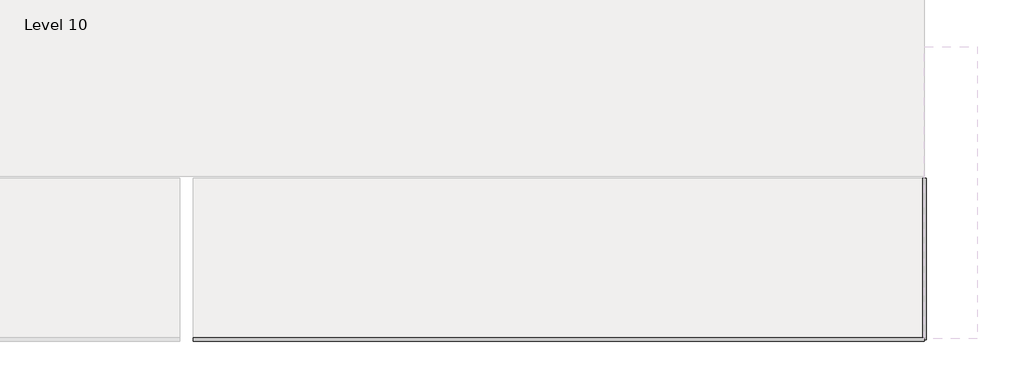
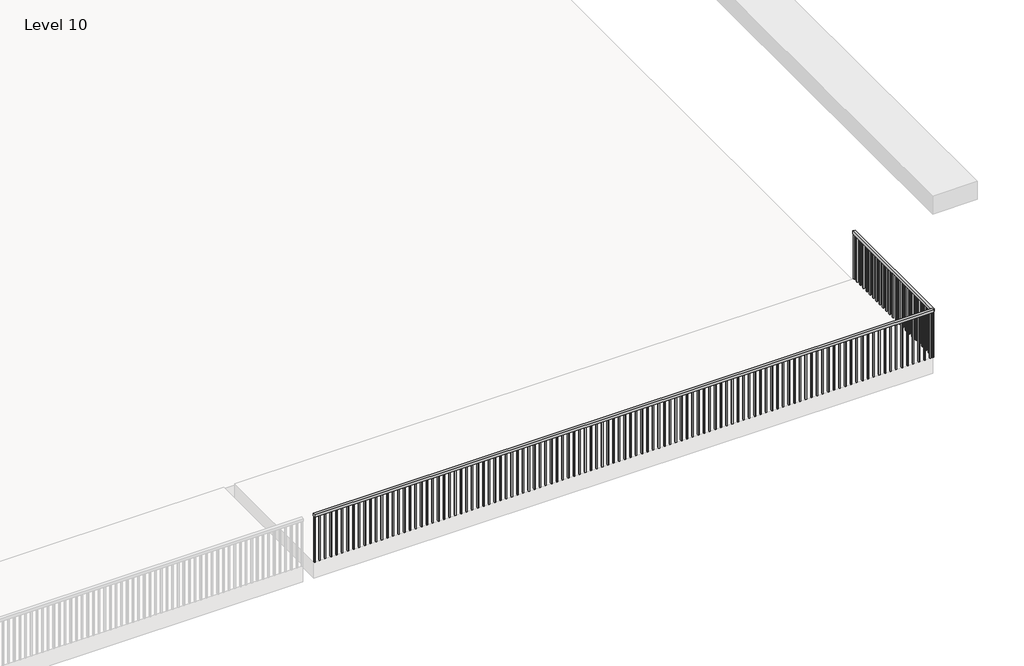
# One storey, part 2 of 5: 2 railings.
"""IFC4 building model written with IfcOpenShell, lengths in millimetres."""

from ifc_helpers import new_model, si_unit, frame, origin, place, context, project, spatial, polyline, outline, extrude, element, save

model = new_model("IFC4")

# Units and contexts
model_context = context("Model", 3, world=origin())
ifc_project = project(units=[si_unit("LENGTHUNIT", "METRE", prefix="MILLI")], contexts=[model_context])

# Site, building, storey
site = spatial("IfcSite", under=ifc_project)
building = spatial("IfcBuilding", under=site)
storey = spatial("IfcBuildingStorey", under=building, Name="Level 10", Elevation=12496.8)

# Railings
placement = place(None, origin())
element("IfcRailing", 1, ObjectType="Handrail - Rectangular", at=placement, inside=storey, context=model_context, shape_type="SweptSolid", body=[
    extrude(outline(polyline([(2981.3361222, -12911.7749501), (2981.3361222, -12860.9749501), (14106.5361222, -12860.9749501), (14106.5361222, -12911.7749501), (2981.3361222, -12911.7749501)])), frame((0.0, 0.0, 13360.4), z_axis=(0.0, 0.0, 1.0), x_axis=(1.0, 0.0, 0.0)), (0.0, 0.0, 1.0), 50.8),
    extrude(outline(polyline([(14046.2111222, -12895.8999501), (14046.2111222, -12876.8499501), (14065.2611222, -12876.8499501), (14065.2611222, -12895.8999501), (14046.2111222, -12895.8999501)])), frame((0.0, 0.0, 12496.8), z_axis=(0.0, 0.0, 1.0), x_axis=(1.0, 0.0, 0.0)), (0.0, 0.0, 1.0), 863.6),
    extrude(outline(polyline([(13944.6111222, -12895.8999501), (13944.6111222, -12876.8499501), (13963.6611222, -12876.8499501), (13963.6611222, -12895.8999501), (13944.6111222, -12895.8999501)])), frame((0.0, 0.0, 12496.8), z_axis=(0.0, 0.0, 1.0), x_axis=(1.0, 0.0, 0.0)), (0.0, 0.0, 1.0), 863.6),
    extrude(outline(polyline([(13843.0111222, -12895.8999501), (13843.0111222, -12876.8499501), (13862.0611222, -12876.8499501), (13862.0611222, -12895.8999501), (13843.0111222, -12895.8999501)])), frame((0.0, 0.0, 12496.8), z_axis=(0.0, 0.0, 1.0), x_axis=(1.0, 0.0, 0.0)), (0.0, 0.0, 1.0), 863.6),
    extrude(outline(polyline([(13741.4111222, -12895.8999501), (13741.4111222, -12876.8499501), (13760.4611222, -12876.8499501), (13760.4611222, -12895.8999501), (13741.4111222, -12895.8999501)])), frame((0.0, 0.0, 12496.8), z_axis=(0.0, 0.0, 1.0), x_axis=(1.0, 0.0, 0.0)), (0.0, 0.0, 1.0), 863.6),
    extrude(outline(polyline([(13639.8111222, -12895.8999501), (13639.8111222, -12876.8499501), (13658.8611222, -12876.8499501), (13658.8611222, -12895.8999501), (13639.8111222, -12895.8999501)])), frame((0.0, 0.0, 12496.8), z_axis=(0.0, 0.0, 1.0), x_axis=(1.0, 0.0, 0.0)), (0.0, 0.0, 1.0), 863.6),
    extrude(outline(polyline([(13538.2111222, -12895.8999501), (13538.2111222, -12876.8499501), (13557.2611222, -12876.8499501), (13557.2611222, -12895.8999501), (13538.2111222, -12895.8999501)])), frame((0.0, 0.0, 12496.8), z_axis=(0.0, 0.0, 1.0), x_axis=(1.0, 0.0, 0.0)), (0.0, 0.0, 1.0), 863.6),
    extrude(outline(polyline([(13436.6111222, -12895.8999501), (13436.6111222, -12876.8499501), (13455.6611222, -12876.8499501), (13455.6611222, -12895.8999501), (13436.6111222, -12895.8999501)])), frame((0.0, 0.0, 12496.8), z_axis=(0.0, 0.0, 1.0), x_axis=(1.0, 0.0, 0.0)), (0.0, 0.0, 1.0), 863.6),
    extrude(outline(polyline([(13335.0111222, -12895.8999501), (13335.0111222, -12876.8499501), (13354.0611222, -12876.8499501), (13354.0611222, -12895.8999501), (13335.0111222, -12895.8999501)])), frame((0.0, 0.0, 12496.8), z_axis=(0.0, 0.0, 1.0), x_axis=(1.0, 0.0, 0.0)), (0.0, 0.0, 1.0), 863.6),
    extrude(outline(polyline([(13233.4111222, -12895.8999501), (13233.4111222, -12876.8499501), (13252.4611222, -12876.8499501), (13252.4611222, -12895.8999501), (13233.4111222, -12895.8999501)])), frame((0.0, 0.0, 12496.8), z_axis=(0.0, 0.0, 1.0), x_axis=(1.0, 0.0, 0.0)), (0.0, 0.0, 1.0), 863.6),
    extrude(outline(polyline([(13131.8111222, -12895.8999501), (13131.8111222, -12876.8499501), (13150.8611222, -12876.8499501), (13150.8611222, -12895.8999501), (13131.8111222, -12895.8999501)])), frame((0.0, 0.0, 12496.8), z_axis=(0.0, 0.0, 1.0), x_axis=(1.0, 0.0, 0.0)), (0.0, 0.0, 1.0), 863.6),
    extrude(outline(polyline([(13030.2111222, -12895.8999501), (13030.2111222, -12876.8499501), (13049.2611222, -12876.8499501), (13049.2611222, -12895.8999501), (13030.2111222, -12895.8999501)])), frame((0.0, 0.0, 12496.8), z_axis=(0.0, 0.0, 1.0), x_axis=(1.0, 0.0, 0.0)), (0.0, 0.0, 1.0), 863.6),
    extrude(outline(polyline([(12928.6111222, -12895.8999501), (12928.6111222, -12876.8499501), (12947.6611222, -12876.8499501), (12947.6611222, -12895.8999501), (12928.6111222, -12895.8999501)])), frame((0.0, 0.0, 12496.8), z_axis=(0.0, 0.0, 1.0), x_axis=(1.0, 0.0, 0.0)), (0.0, 0.0, 1.0), 863.6),
    extrude(outline(polyline([(12827.0111222, -12895.8999501), (12827.0111222, -12876.8499501), (12846.0611222, -12876.8499501), (12846.0611222, -12895.8999501), (12827.0111222, -12895.8999501)])), frame((0.0, 0.0, 12496.8), z_axis=(0.0, 0.0, 1.0), x_axis=(1.0, 0.0, 0.0)), (0.0, 0.0, 1.0), 863.6),
    extrude(outline(polyline([(12725.4111222, -12895.8999501), (12725.4111222, -12876.8499501), (12744.4611222, -12876.8499501), (12744.4611222, -12895.8999501), (12725.4111222, -12895.8999501)])), frame((0.0, 0.0, 12496.8), z_axis=(0.0, 0.0, 1.0), x_axis=(1.0, 0.0, 0.0)), (0.0, 0.0, 1.0), 863.6),
    extrude(outline(polyline([(12623.8111222, -12895.8999501), (12623.8111222, -12876.8499501), (12642.8611222, -12876.8499501), (12642.8611222, -12895.8999501), (12623.8111222, -12895.8999501)])), frame((0.0, 0.0, 12496.8), z_axis=(0.0, 0.0, 1.0), x_axis=(1.0, 0.0, 0.0)), (0.0, 0.0, 1.0), 863.6),
    extrude(outline(polyline([(12522.2111222, -12895.8999501), (12522.2111222, -12876.8499501), (12541.2611222, -12876.8499501), (12541.2611222, -12895.8999501), (12522.2111222, -12895.8999501)])), frame((0.0, 0.0, 12496.8), z_axis=(0.0, 0.0, 1.0), x_axis=(1.0, 0.0, 0.0)), (0.0, 0.0, 1.0), 863.6),
    extrude(outline(polyline([(12420.6111222, -12895.8999501), (12420.6111222, -12876.8499501), (12439.6611222, -12876.8499501), (12439.6611222, -12895.8999501), (12420.6111222, -12895.8999501)])), frame((0.0, 0.0, 12496.8), z_axis=(0.0, 0.0, 1.0), x_axis=(1.0, 0.0, 0.0)), (0.0, 0.0, 1.0), 863.6),
    extrude(outline(polyline([(12319.0111222, -12895.8999501), (12319.0111222, -12876.8499501), (12338.0611222, -12876.8499501), (12338.0611222, -12895.8999501), (12319.0111222, -12895.8999501)])), frame((0.0, 0.0, 12496.8), z_axis=(0.0, 0.0, 1.0), x_axis=(1.0, 0.0, 0.0)), (0.0, 0.0, 1.0), 863.6),
    extrude(outline(polyline([(12217.4111222, -12895.8999501), (12217.4111222, -12876.8499501), (12236.4611222, -12876.8499501), (12236.4611222, -12895.8999501), (12217.4111222, -12895.8999501)])), frame((0.0, 0.0, 12496.8), z_axis=(0.0, 0.0, 1.0), x_axis=(1.0, 0.0, 0.0)), (0.0, 0.0, 1.0), 863.6),
    extrude(outline(polyline([(12115.8111222, -12895.8999501), (12115.8111222, -12876.8499501), (12134.8611222, -12876.8499501), (12134.8611222, -12895.8999501), (12115.8111222, -12895.8999501)])), frame((0.0, 0.0, 12496.8), z_axis=(0.0, 0.0, 1.0), x_axis=(1.0, 0.0, 0.0)), (0.0, 0.0, 1.0), 863.6),
    extrude(outline(polyline([(12014.2111222, -12895.8999501), (12014.2111222, -12876.8499501), (12033.2611222, -12876.8499501), (12033.2611222, -12895.8999501), (12014.2111222, -12895.8999501)])), frame((0.0, 0.0, 12496.8), z_axis=(0.0, 0.0, 1.0), x_axis=(1.0, 0.0, 0.0)), (0.0, 0.0, 1.0), 863.6),
    extrude(outline(polyline([(11912.6111222, -12895.8999501), (11912.6111222, -12876.8499501), (11931.6611222, -12876.8499501), (11931.6611222, -12895.8999501), (11912.6111222, -12895.8999501)])), frame((0.0, 0.0, 12496.8), z_axis=(0.0, 0.0, 1.0), x_axis=(1.0, 0.0, 0.0)), (0.0, 0.0, 1.0), 863.6),
    extrude(outline(polyline([(11811.0111222, -12895.8999501), (11811.0111222, -12876.8499501), (11830.0611222, -12876.8499501), (11830.0611222, -12895.8999501), (11811.0111222, -12895.8999501)])), frame((0.0, 0.0, 12496.8), z_axis=(0.0, 0.0, 1.0), x_axis=(1.0, 0.0, 0.0)), (0.0, 0.0, 1.0), 863.6),
    extrude(outline(polyline([(11709.4111222, -12895.8999501), (11709.4111222, -12876.8499501), (11728.4611222, -12876.8499501), (11728.4611222, -12895.8999501), (11709.4111222, -12895.8999501)])), frame((0.0, 0.0, 12496.8), z_axis=(0.0, 0.0, 1.0), x_axis=(1.0, 0.0, 0.0)), (0.0, 0.0, 1.0), 863.6),
    extrude(outline(polyline([(11607.8111222, -12895.8999501), (11607.8111222, -12876.8499501), (11626.8611222, -12876.8499501), (11626.8611222, -12895.8999501), (11607.8111222, -12895.8999501)])), frame((0.0, 0.0, 12496.8), z_axis=(0.0, 0.0, 1.0), x_axis=(1.0, 0.0, 0.0)), (0.0, 0.0, 1.0), 863.6),
    extrude(outline(polyline([(11506.2111222, -12895.8999501), (11506.2111222, -12876.8499501), (11525.2611222, -12876.8499501), (11525.2611222, -12895.8999501), (11506.2111222, -12895.8999501)])), frame((0.0, 0.0, 12496.8), z_axis=(0.0, 0.0, 1.0), x_axis=(1.0, 0.0, 0.0)), (0.0, 0.0, 1.0), 863.6),
    extrude(outline(polyline([(11404.6111222, -12895.8999501), (11404.6111222, -12876.8499501), (11423.6611222, -12876.8499501), (11423.6611222, -12895.8999501), (11404.6111222, -12895.8999501)])), frame((0.0, 0.0, 12496.8), z_axis=(0.0, 0.0, 1.0), x_axis=(1.0, 0.0, 0.0)), (0.0, 0.0, 1.0), 863.6),
    extrude(outline(polyline([(11303.0111222, -12895.8999501), (11303.0111222, -12876.8499501), (11322.0611222, -12876.8499501), (11322.0611222, -12895.8999501), (11303.0111222, -12895.8999501)])), frame((0.0, 0.0, 12496.8), z_axis=(0.0, 0.0, 1.0), x_axis=(1.0, 0.0, 0.0)), (0.0, 0.0, 1.0), 863.6),
    extrude(outline(polyline([(11201.4111222, -12895.8999501), (11201.4111222, -12876.8499501), (11220.4611222, -12876.8499501), (11220.4611222, -12895.8999501), (11201.4111222, -12895.8999501)])), frame((0.0, 0.0, 12496.8), z_axis=(0.0, 0.0, 1.0), x_axis=(1.0, 0.0, 0.0)), (0.0, 0.0, 1.0), 863.6),
    extrude(outline(polyline([(11099.8111222, -12895.8999501), (11099.8111222, -12876.8499501), (11118.8611222, -12876.8499501), (11118.8611222, -12895.8999501), (11099.8111222, -12895.8999501)])), frame((0.0, 0.0, 12496.8), z_axis=(0.0, 0.0, 1.0), x_axis=(1.0, 0.0, 0.0)), (0.0, 0.0, 1.0), 863.6),
    extrude(outline(polyline([(10998.2111222, -12895.8999501), (10998.2111222, -12876.8499501), (11017.2611222, -12876.8499501), (11017.2611222, -12895.8999501), (10998.2111222, -12895.8999501)])), frame((0.0, 0.0, 12496.8), z_axis=(0.0, 0.0, 1.0), x_axis=(1.0, 0.0, 0.0)), (0.0, 0.0, 1.0), 863.6),
    extrude(outline(polyline([(10896.6111222, -12895.8999501), (10896.6111222, -12876.8499501), (10915.6611222, -12876.8499501), (10915.6611222, -12895.8999501), (10896.6111222, -12895.8999501)])), frame((0.0, 0.0, 12496.8), z_axis=(0.0, 0.0, 1.0), x_axis=(1.0, 0.0, 0.0)), (0.0, 0.0, 1.0), 863.6),
    extrude(outline(polyline([(10795.0111222, -12895.8999501), (10795.0111222, -12876.8499501), (10814.0611222, -12876.8499501), (10814.0611222, -12895.8999501), (10795.0111222, -12895.8999501)])), frame((0.0, 0.0, 12496.8), z_axis=(0.0, 0.0, 1.0), x_axis=(1.0, 0.0, 0.0)), (0.0, 0.0, 1.0), 863.6),
    extrude(outline(polyline([(10693.4111222, -12895.8999501), (10693.4111222, -12876.8499501), (10712.4611222, -12876.8499501), (10712.4611222, -12895.8999501), (10693.4111222, -12895.8999501)])), frame((0.0, 0.0, 12496.8), z_axis=(0.0, 0.0, 1.0), x_axis=(1.0, 0.0, 0.0)), (0.0, 0.0, 1.0), 863.6),
    extrude(outline(polyline([(10591.8111222, -12895.8999501), (10591.8111222, -12876.8499501), (10610.8611222, -12876.8499501), (10610.8611222, -12895.8999501), (10591.8111222, -12895.8999501)])), frame((0.0, 0.0, 12496.8), z_axis=(0.0, 0.0, 1.0), x_axis=(1.0, 0.0, 0.0)), (0.0, 0.0, 1.0), 863.6),
    extrude(outline(polyline([(10490.2111222, -12895.8999501), (10490.2111222, -12876.8499501), (10509.2611222, -12876.8499501), (10509.2611222, -12895.8999501), (10490.2111222, -12895.8999501)])), frame((0.0, 0.0, 12496.8), z_axis=(0.0, 0.0, 1.0), x_axis=(1.0, 0.0, 0.0)), (0.0, 0.0, 1.0), 863.6),
    extrude(outline(polyline([(10388.6111222, -12895.8999501), (10388.6111222, -12876.8499501), (10407.6611222, -12876.8499501), (10407.6611222, -12895.8999501), (10388.6111222, -12895.8999501)])), frame((0.0, 0.0, 12496.8), z_axis=(0.0, 0.0, 1.0), x_axis=(1.0, 0.0, 0.0)), (0.0, 0.0, 1.0), 863.6),
    extrude(outline(polyline([(10287.0111222, -12895.8999501), (10287.0111222, -12876.8499501), (10306.0611222, -12876.8499501), (10306.0611222, -12895.8999501), (10287.0111222, -12895.8999501)])), frame((0.0, 0.0, 12496.8), z_axis=(0.0, 0.0, 1.0), x_axis=(1.0, 0.0, 0.0)), (0.0, 0.0, 1.0), 863.6),
    extrude(outline(polyline([(10185.4111222, -12895.8999501), (10185.4111222, -12876.8499501), (10204.4611222, -12876.8499501), (10204.4611222, -12895.8999501), (10185.4111222, -12895.8999501)])), frame((0.0, 0.0, 12496.8), z_axis=(0.0, 0.0, 1.0), x_axis=(1.0, 0.0, 0.0)), (0.0, 0.0, 1.0), 863.6),
    extrude(outline(polyline([(10083.8111222, -12895.8999501), (10083.8111222, -12876.8499501), (10102.8611222, -12876.8499501), (10102.8611222, -12895.8999501), (10083.8111222, -12895.8999501)])), frame((0.0, 0.0, 12496.8), z_axis=(0.0, 0.0, 1.0), x_axis=(1.0, 0.0, 0.0)), (0.0, 0.0, 1.0), 863.6),
    extrude(outline(polyline([(9982.2111222, -12895.8999501), (9982.2111222, -12876.8499501), (10001.2611222, -12876.8499501), (10001.2611222, -12895.8999501), (9982.2111222, -12895.8999501)])), frame((0.0, 0.0, 12496.8), z_axis=(0.0, 0.0, 1.0), x_axis=(1.0, 0.0, 0.0)), (0.0, 0.0, 1.0), 863.6),
    extrude(outline(polyline([(9880.6111222, -12895.8999501), (9880.6111222, -12876.8499501), (9899.6611222, -12876.8499501), (9899.6611222, -12895.8999501), (9880.6111222, -12895.8999501)])), frame((0.0, 0.0, 12496.8), z_axis=(0.0, 0.0, 1.0), x_axis=(1.0, 0.0, 0.0)), (0.0, 0.0, 1.0), 863.6),
    extrude(outline(polyline([(9779.0111222, -12895.8999501), (9779.0111222, -12876.8499501), (9798.0611222, -12876.8499501), (9798.0611222, -12895.8999501), (9779.0111222, -12895.8999501)])), frame((0.0, 0.0, 12496.8), z_axis=(0.0, 0.0, 1.0), x_axis=(1.0, 0.0, 0.0)), (0.0, 0.0, 1.0), 863.6),
    extrude(outline(polyline([(9677.4111222, -12895.8999501), (9677.4111222, -12876.8499501), (9696.4611222, -12876.8499501), (9696.4611222, -12895.8999501), (9677.4111222, -12895.8999501)])), frame((0.0, 0.0, 12496.8), z_axis=(0.0, 0.0, 1.0), x_axis=(1.0, 0.0, 0.0)), (0.0, 0.0, 1.0), 863.6),
    extrude(outline(polyline([(9575.8111222, -12895.8999501), (9575.8111222, -12876.8499501), (9594.8611222, -12876.8499501), (9594.8611222, -12895.8999501), (9575.8111222, -12895.8999501)])), frame((0.0, 0.0, 12496.8), z_axis=(0.0, 0.0, 1.0), x_axis=(1.0, 0.0, 0.0)), (0.0, 0.0, 1.0), 863.6),
    extrude(outline(polyline([(9474.2111222, -12895.8999501), (9474.2111222, -12876.8499501), (9493.2611222, -12876.8499501), (9493.2611222, -12895.8999501), (9474.2111222, -12895.8999501)])), frame((0.0, 0.0, 12496.8), z_axis=(0.0, 0.0, 1.0), x_axis=(1.0, 0.0, 0.0)), (0.0, 0.0, 1.0), 863.6),
    extrude(outline(polyline([(9372.6111222, -12895.8999501), (9372.6111222, -12876.8499501), (9391.6611222, -12876.8499501), (9391.6611222, -12895.8999501), (9372.6111222, -12895.8999501)])), frame((0.0, 0.0, 12496.8), z_axis=(0.0, 0.0, 1.0), x_axis=(1.0, 0.0, 0.0)), (0.0, 0.0, 1.0), 863.6),
    extrude(outline(polyline([(9271.0111222, -12895.8999501), (9271.0111222, -12876.8499501), (9290.0611222, -12876.8499501), (9290.0611222, -12895.8999501), (9271.0111222, -12895.8999501)])), frame((0.0, 0.0, 12496.8), z_axis=(0.0, 0.0, 1.0), x_axis=(1.0, 0.0, 0.0)), (0.0, 0.0, 1.0), 863.6),
    extrude(outline(polyline([(9169.4111222, -12895.8999501), (9169.4111222, -12876.8499501), (9188.4611222, -12876.8499501), (9188.4611222, -12895.8999501), (9169.4111222, -12895.8999501)])), frame((0.0, 0.0, 12496.8), z_axis=(0.0, 0.0, 1.0), x_axis=(1.0, 0.0, 0.0)), (0.0, 0.0, 1.0), 863.6),
    extrude(outline(polyline([(9067.8111222, -12895.8999501), (9067.8111222, -12876.8499501), (9086.8611222, -12876.8499501), (9086.8611222, -12895.8999501), (9067.8111222, -12895.8999501)])), frame((0.0, 0.0, 12496.8), z_axis=(0.0, 0.0, 1.0), x_axis=(1.0, 0.0, 0.0)), (0.0, 0.0, 1.0), 863.6),
    extrude(outline(polyline([(8966.2111222, -12895.8999501), (8966.2111222, -12876.8499501), (8985.2611222, -12876.8499501), (8985.2611222, -12895.8999501), (8966.2111222, -12895.8999501)])), frame((0.0, 0.0, 12496.8), z_axis=(0.0, 0.0, 1.0), x_axis=(1.0, 0.0, 0.0)), (0.0, 0.0, 1.0), 863.6),
    extrude(outline(polyline([(8864.6111222, -12895.8999501), (8864.6111222, -12876.8499501), (8883.6611222, -12876.8499501), (8883.6611222, -12895.8999501), (8864.6111222, -12895.8999501)])), frame((0.0, 0.0, 12496.8), z_axis=(0.0, 0.0, 1.0), x_axis=(1.0, 0.0, 0.0)), (0.0, 0.0, 1.0), 863.6),
    extrude(outline(polyline([(8763.0111222, -12895.8999501), (8763.0111222, -12876.8499501), (8782.0611222, -12876.8499501), (8782.0611222, -12895.8999501), (8763.0111222, -12895.8999501)])), frame((0.0, 0.0, 12496.8), z_axis=(0.0, 0.0, 1.0), x_axis=(1.0, 0.0, 0.0)), (0.0, 0.0, 1.0), 863.6),
    extrude(outline(polyline([(8661.4111222, -12895.8999501), (8661.4111222, -12876.8499501), (8680.4611222, -12876.8499501), (8680.4611222, -12895.8999501), (8661.4111222, -12895.8999501)])), frame((0.0, 0.0, 12496.8), z_axis=(0.0, 0.0, 1.0), x_axis=(1.0, 0.0, 0.0)), (0.0, 0.0, 1.0), 863.6),
    extrude(outline(polyline([(8559.8111222, -12895.8999501), (8559.8111222, -12876.8499501), (8578.8611222, -12876.8499501), (8578.8611222, -12895.8999501), (8559.8111222, -12895.8999501)])), frame((0.0, 0.0, 12496.8), z_axis=(0.0, 0.0, 1.0), x_axis=(1.0, 0.0, 0.0)), (0.0, 0.0, 1.0), 863.6),
    extrude(outline(polyline([(8458.2111222, -12895.8999501), (8458.2111222, -12876.8499501), (8477.2611222, -12876.8499501), (8477.2611222, -12895.8999501), (8458.2111222, -12895.8999501)])), frame((0.0, 0.0, 12496.8), z_axis=(0.0, 0.0, 1.0), x_axis=(1.0, 0.0, 0.0)), (0.0, 0.0, 1.0), 863.6),
    extrude(outline(polyline([(8356.6111222, -12895.8999501), (8356.6111222, -12876.8499501), (8375.6611222, -12876.8499501), (8375.6611222, -12895.8999501), (8356.6111222, -12895.8999501)])), frame((0.0, 0.0, 12496.8), z_axis=(0.0, 0.0, 1.0), x_axis=(1.0, 0.0, 0.0)), (0.0, 0.0, 1.0), 863.6),
    extrude(outline(polyline([(8255.0111222, -12895.8999501), (8255.0111222, -12876.8499501), (8274.0611222, -12876.8499501), (8274.0611222, -12895.8999501), (8255.0111222, -12895.8999501)])), frame((0.0, 0.0, 12496.8), z_axis=(0.0, 0.0, 1.0), x_axis=(1.0, 0.0, 0.0)), (0.0, 0.0, 1.0), 863.6),
    extrude(outline(polyline([(8153.4111222, -12895.8999501), (8153.4111222, -12876.8499501), (8172.4611222, -12876.8499501), (8172.4611222, -12895.8999501), (8153.4111222, -12895.8999501)])), frame((0.0, 0.0, 12496.8), z_axis=(0.0, 0.0, 1.0), x_axis=(1.0, 0.0, 0.0)), (0.0, 0.0, 1.0), 863.6),
    extrude(outline(polyline([(8051.8111222, -12895.8999501), (8051.8111222, -12876.8499501), (8070.8611222, -12876.8499501), (8070.8611222, -12895.8999501), (8051.8111222, -12895.8999501)])), frame((0.0, 0.0, 12496.8), z_axis=(0.0, 0.0, 1.0), x_axis=(1.0, 0.0, 0.0)), (0.0, 0.0, 1.0), 863.6),
    extrude(outline(polyline([(7950.2111222, -12895.8999501), (7950.2111222, -12876.8499501), (7969.2611222, -12876.8499501), (7969.2611222, -12895.8999501), (7950.2111222, -12895.8999501)])), frame((0.0, 0.0, 12496.8), z_axis=(0.0, 0.0, 1.0), x_axis=(1.0, 0.0, 0.0)), (0.0, 0.0, 1.0), 863.6),
    extrude(outline(polyline([(7848.6111222, -12895.8999501), (7848.6111222, -12876.8499501), (7867.6611222, -12876.8499501), (7867.6611222, -12895.8999501), (7848.6111222, -12895.8999501)])), frame((0.0, 0.0, 12496.8), z_axis=(0.0, 0.0, 1.0), x_axis=(1.0, 0.0, 0.0)), (0.0, 0.0, 1.0), 863.6),
    extrude(outline(polyline([(7747.0111222, -12895.8999501), (7747.0111222, -12876.8499501), (7766.0611222, -12876.8499501), (7766.0611222, -12895.8999501), (7747.0111222, -12895.8999501)])), frame((0.0, 0.0, 12496.8), z_axis=(0.0, 0.0, 1.0), x_axis=(1.0, 0.0, 0.0)), (0.0, 0.0, 1.0), 863.6),
    extrude(outline(polyline([(7645.4111222, -12895.8999501), (7645.4111222, -12876.8499501), (7664.4611222, -12876.8499501), (7664.4611222, -12895.8999501), (7645.4111222, -12895.8999501)])), frame((0.0, 0.0, 12496.8), z_axis=(0.0, 0.0, 1.0), x_axis=(1.0, 0.0, 0.0)), (0.0, 0.0, 1.0), 863.6),
    extrude(outline(polyline([(7543.8111222, -12895.8999501), (7543.8111222, -12876.8499501), (7562.8611222, -12876.8499501), (7562.8611222, -12895.8999501), (7543.8111222, -12895.8999501)])), frame((0.0, 0.0, 12496.8), z_axis=(0.0, 0.0, 1.0), x_axis=(1.0, 0.0, 0.0)), (0.0, 0.0, 1.0), 863.6),
    extrude(outline(polyline([(7442.2111222, -12895.8999501), (7442.2111222, -12876.8499501), (7461.2611222, -12876.8499501), (7461.2611222, -12895.8999501), (7442.2111222, -12895.8999501)])), frame((0.0, 0.0, 12496.8), z_axis=(0.0, 0.0, 1.0), x_axis=(1.0, 0.0, 0.0)), (0.0, 0.0, 1.0), 863.6),
    extrude(outline(polyline([(7340.6111222, -12895.8999501), (7340.6111222, -12876.8499501), (7359.6611222, -12876.8499501), (7359.6611222, -12895.8999501), (7340.6111222, -12895.8999501)])), frame((0.0, 0.0, 12496.8), z_axis=(0.0, 0.0, 1.0), x_axis=(1.0, 0.0, 0.0)), (0.0, 0.0, 1.0), 863.6),
    extrude(outline(polyline([(7239.0111222, -12895.8999501), (7239.0111222, -12876.8499501), (7258.0611222, -12876.8499501), (7258.0611222, -12895.8999501), (7239.0111222, -12895.8999501)])), frame((0.0, 0.0, 12496.8), z_axis=(0.0, 0.0, 1.0), x_axis=(1.0, 0.0, 0.0)), (0.0, 0.0, 1.0), 863.6),
    extrude(outline(polyline([(7137.4111222, -12895.8999501), (7137.4111222, -12876.8499501), (7156.4611222, -12876.8499501), (7156.4611222, -12895.8999501), (7137.4111222, -12895.8999501)])), frame((0.0, 0.0, 12496.8), z_axis=(0.0, 0.0, 1.0), x_axis=(1.0, 0.0, 0.0)), (0.0, 0.0, 1.0), 863.6),
    extrude(outline(polyline([(7035.8111222, -12895.8999501), (7035.8111222, -12876.8499501), (7054.8611222, -12876.8499501), (7054.8611222, -12895.8999501), (7035.8111222, -12895.8999501)])), frame((0.0, 0.0, 12496.8), z_axis=(0.0, 0.0, 1.0), x_axis=(1.0, 0.0, 0.0)), (0.0, 0.0, 1.0), 863.6),
    extrude(outline(polyline([(6934.2111222, -12895.8999501), (6934.2111222, -12876.8499501), (6953.2611222, -12876.8499501), (6953.2611222, -12895.8999501), (6934.2111222, -12895.8999501)])), frame((0.0, 0.0, 12496.8), z_axis=(0.0, 0.0, 1.0), x_axis=(1.0, 0.0, 0.0)), (0.0, 0.0, 1.0), 863.6),
    extrude(outline(polyline([(6832.6111222, -12895.8999501), (6832.6111222, -12876.8499501), (6851.6611222, -12876.8499501), (6851.6611222, -12895.8999501), (6832.6111222, -12895.8999501)])), frame((0.0, 0.0, 12496.8), z_axis=(0.0, 0.0, 1.0), x_axis=(1.0, 0.0, 0.0)), (0.0, 0.0, 1.0), 863.6),
    extrude(outline(polyline([(6731.0111222, -12895.8999501), (6731.0111222, -12876.8499501), (6750.0611222, -12876.8499501), (6750.0611222, -12895.8999501), (6731.0111222, -12895.8999501)])), frame((0.0, 0.0, 12496.8), z_axis=(0.0, 0.0, 1.0), x_axis=(1.0, 0.0, 0.0)), (0.0, 0.0, 1.0), 863.6),
    extrude(outline(polyline([(6629.4111222, -12895.8999501), (6629.4111222, -12876.8499501), (6648.4611222, -12876.8499501), (6648.4611222, -12895.8999501), (6629.4111222, -12895.8999501)])), frame((0.0, 0.0, 12496.8), z_axis=(0.0, 0.0, 1.0), x_axis=(1.0, 0.0, 0.0)), (0.0, 0.0, 1.0), 863.6),
    extrude(outline(polyline([(6527.8111222, -12895.8999501), (6527.8111222, -12876.8499501), (6546.8611222, -12876.8499501), (6546.8611222, -12895.8999501), (6527.8111222, -12895.8999501)])), frame((0.0, 0.0, 12496.8), z_axis=(0.0, 0.0, 1.0), x_axis=(1.0, 0.0, 0.0)), (0.0, 0.0, 1.0), 863.6),
    extrude(outline(polyline([(6426.2111222, -12895.8999501), (6426.2111222, -12876.8499501), (6445.2611222, -12876.8499501), (6445.2611222, -12895.8999501), (6426.2111222, -12895.8999501)])), frame((0.0, 0.0, 12496.8), z_axis=(0.0, 0.0, 1.0), x_axis=(1.0, 0.0, 0.0)), (0.0, 0.0, 1.0), 863.6),
    extrude(outline(polyline([(6324.6111222, -12895.8999501), (6324.6111222, -12876.8499501), (6343.6611222, -12876.8499501), (6343.6611222, -12895.8999501), (6324.6111222, -12895.8999501)])), frame((0.0, 0.0, 12496.8), z_axis=(0.0, 0.0, 1.0), x_axis=(1.0, 0.0, 0.0)), (0.0, 0.0, 1.0), 863.6),
    extrude(outline(polyline([(6223.0111222, -12895.8999501), (6223.0111222, -12876.8499501), (6242.0611222, -12876.8499501), (6242.0611222, -12895.8999501), (6223.0111222, -12895.8999501)])), frame((0.0, 0.0, 12496.8), z_axis=(0.0, 0.0, 1.0), x_axis=(1.0, 0.0, 0.0)), (0.0, 0.0, 1.0), 863.6),
    extrude(outline(polyline([(6121.4111222, -12895.8999501), (6121.4111222, -12876.8499501), (6140.4611222, -12876.8499501), (6140.4611222, -12895.8999501), (6121.4111222, -12895.8999501)])), frame((0.0, 0.0, 12496.8), z_axis=(0.0, 0.0, 1.0), x_axis=(1.0, 0.0, 0.0)), (0.0, 0.0, 1.0), 863.6),
    extrude(outline(polyline([(6019.8111222, -12895.8999501), (6019.8111222, -12876.8499501), (6038.8611222, -12876.8499501), (6038.8611222, -12895.8999501), (6019.8111222, -12895.8999501)])), frame((0.0, 0.0, 12496.8), z_axis=(0.0, 0.0, 1.0), x_axis=(1.0, 0.0, 0.0)), (0.0, 0.0, 1.0), 863.6),
    extrude(outline(polyline([(5918.2111222, -12895.8999501), (5918.2111222, -12876.8499501), (5937.2611222, -12876.8499501), (5937.2611222, -12895.8999501), (5918.2111222, -12895.8999501)])), frame((0.0, 0.0, 12496.8), z_axis=(0.0, 0.0, 1.0), x_axis=(1.0, 0.0, 0.0)), (0.0, 0.0, 1.0), 863.6),
    extrude(outline(polyline([(5816.6111222, -12895.8999501), (5816.6111222, -12876.8499501), (5835.6611222, -12876.8499501), (5835.6611222, -12895.8999501), (5816.6111222, -12895.8999501)])), frame((0.0, 0.0, 12496.8), z_axis=(0.0, 0.0, 1.0), x_axis=(1.0, 0.0, 0.0)), (0.0, 0.0, 1.0), 863.6),
    extrude(outline(polyline([(5715.0111222, -12895.8999501), (5715.0111222, -12876.8499501), (5734.0611222, -12876.8499501), (5734.0611222, -12895.8999501), (5715.0111222, -12895.8999501)])), frame((0.0, 0.0, 12496.8), z_axis=(0.0, 0.0, 1.0), x_axis=(1.0, 0.0, 0.0)), (0.0, 0.0, 1.0), 863.6),
    extrude(outline(polyline([(5613.4111222, -12895.8999501), (5613.4111222, -12876.8499501), (5632.4611222, -12876.8499501), (5632.4611222, -12895.8999501), (5613.4111222, -12895.8999501)])), frame((0.0, 0.0, 12496.8), z_axis=(0.0, 0.0, 1.0), x_axis=(1.0, 0.0, 0.0)), (0.0, 0.0, 1.0), 863.6),
    extrude(outline(polyline([(5511.8111222, -12895.8999501), (5511.8111222, -12876.8499501), (5530.8611222, -12876.8499501), (5530.8611222, -12895.8999501), (5511.8111222, -12895.8999501)])), frame((0.0, 0.0, 12496.8), z_axis=(0.0, 0.0, 1.0), x_axis=(1.0, 0.0, 0.0)), (0.0, 0.0, 1.0), 863.6),
    extrude(outline(polyline([(5410.2111222, -12895.8999501), (5410.2111222, -12876.8499501), (5429.2611222, -12876.8499501), (5429.2611222, -12895.8999501), (5410.2111222, -12895.8999501)])), frame((0.0, 0.0, 12496.8), z_axis=(0.0, 0.0, 1.0), x_axis=(1.0, 0.0, 0.0)), (0.0, 0.0, 1.0), 863.6),
    extrude(outline(polyline([(5308.6111222, -12895.8999501), (5308.6111222, -12876.8499501), (5327.6611222, -12876.8499501), (5327.6611222, -12895.8999501), (5308.6111222, -12895.8999501)])), frame((0.0, 0.0, 12496.8), z_axis=(0.0, 0.0, 1.0), x_axis=(1.0, 0.0, 0.0)), (0.0, 0.0, 1.0), 863.6),
    extrude(outline(polyline([(5207.0111222, -12895.8999501), (5207.0111222, -12876.8499501), (5226.0611222, -12876.8499501), (5226.0611222, -12895.8999501), (5207.0111222, -12895.8999501)])), frame((0.0, 0.0, 12496.8), z_axis=(0.0, 0.0, 1.0), x_axis=(1.0, 0.0, 0.0)), (0.0, 0.0, 1.0), 863.6),
    extrude(outline(polyline([(5105.4111222, -12895.8999501), (5105.4111222, -12876.8499501), (5124.4611222, -12876.8499501), (5124.4611222, -12895.8999501), (5105.4111222, -12895.8999501)])), frame((0.0, 0.0, 12496.8), z_axis=(0.0, 0.0, 1.0), x_axis=(1.0, 0.0, 0.0)), (0.0, 0.0, 1.0), 863.6),
    extrude(outline(polyline([(5003.8111222, -12895.8999501), (5003.8111222, -12876.8499501), (5022.8611222, -12876.8499501), (5022.8611222, -12895.8999501), (5003.8111222, -12895.8999501)])), frame((0.0, 0.0, 12496.8), z_axis=(0.0, 0.0, 1.0), x_axis=(1.0, 0.0, 0.0)), (0.0, 0.0, 1.0), 863.6),
    extrude(outline(polyline([(4902.2111222, -12895.8999501), (4902.2111222, -12876.8499501), (4921.2611222, -12876.8499501), (4921.2611222, -12895.8999501), (4902.2111222, -12895.8999501)])), frame((0.0, 0.0, 12496.8), z_axis=(0.0, 0.0, 1.0), x_axis=(1.0, 0.0, 0.0)), (0.0, 0.0, 1.0), 863.6),
    extrude(outline(polyline([(4800.6111222, -12895.8999501), (4800.6111222, -12876.8499501), (4819.6611222, -12876.8499501), (4819.6611222, -12895.8999501), (4800.6111222, -12895.8999501)])), frame((0.0, 0.0, 12496.8), z_axis=(0.0, 0.0, 1.0), x_axis=(1.0, 0.0, 0.0)), (0.0, 0.0, 1.0), 863.6),
    extrude(outline(polyline([(4699.0111222, -12895.8999501), (4699.0111222, -12876.8499501), (4718.0611222, -12876.8499501), (4718.0611222, -12895.8999501), (4699.0111222, -12895.8999501)])), frame((0.0, 0.0, 12496.8), z_axis=(0.0, 0.0, 1.0), x_axis=(1.0, 0.0, 0.0)), (0.0, 0.0, 1.0), 863.6),
    extrude(outline(polyline([(4597.4111222, -12895.8999501), (4597.4111222, -12876.8499501), (4616.4611222, -12876.8499501), (4616.4611222, -12895.8999501), (4597.4111222, -12895.8999501)])), frame((0.0, 0.0, 12496.8), z_axis=(0.0, 0.0, 1.0), x_axis=(1.0, 0.0, 0.0)), (0.0, 0.0, 1.0), 863.6),
    extrude(outline(polyline([(4495.8111222, -12895.8999501), (4495.8111222, -12876.8499501), (4514.8611222, -12876.8499501), (4514.8611222, -12895.8999501), (4495.8111222, -12895.8999501)])), frame((0.0, 0.0, 12496.8), z_axis=(0.0, 0.0, 1.0), x_axis=(1.0, 0.0, 0.0)), (0.0, 0.0, 1.0), 863.6),
    extrude(outline(polyline([(4394.2111222, -12895.8999501), (4394.2111222, -12876.8499501), (4413.2611222, -12876.8499501), (4413.2611222, -12895.8999501), (4394.2111222, -12895.8999501)])), frame((0.0, 0.0, 12496.8), z_axis=(0.0, 0.0, 1.0), x_axis=(1.0, 0.0, 0.0)), (0.0, 0.0, 1.0), 863.6),
    extrude(outline(polyline([(4292.6111222, -12895.8999501), (4292.6111222, -12876.8499501), (4311.6611222, -12876.8499501), (4311.6611222, -12895.8999501), (4292.6111222, -12895.8999501)])), frame((0.0, 0.0, 12496.8), z_axis=(0.0, 0.0, 1.0), x_axis=(1.0, 0.0, 0.0)), (0.0, 0.0, 1.0), 863.6),
    extrude(outline(polyline([(4191.0111222, -12895.8999501), (4191.0111222, -12876.8499501), (4210.0611222, -12876.8499501), (4210.0611222, -12895.8999501), (4191.0111222, -12895.8999501)])), frame((0.0, 0.0, 12496.8), z_axis=(0.0, 0.0, 1.0), x_axis=(1.0, 0.0, 0.0)), (0.0, 0.0, 1.0), 863.6),
    extrude(outline(polyline([(4089.4111222, -12895.8999501), (4089.4111222, -12876.8499501), (4108.4611222, -12876.8499501), (4108.4611222, -12895.8999501), (4089.4111222, -12895.8999501)])), frame((0.0, 0.0, 12496.8), z_axis=(0.0, 0.0, 1.0), x_axis=(1.0, 0.0, 0.0)), (0.0, 0.0, 1.0), 863.6),
    extrude(outline(polyline([(3987.8111222, -12895.8999501), (3987.8111222, -12876.8499501), (4006.8611222, -12876.8499501), (4006.8611222, -12895.8999501), (3987.8111222, -12895.8999501)])), frame((0.0, 0.0, 12496.8), z_axis=(0.0, 0.0, 1.0), x_axis=(1.0, 0.0, 0.0)), (0.0, 0.0, 1.0), 863.6),
    extrude(outline(polyline([(3886.2111222, -12895.8999501), (3886.2111222, -12876.8499501), (3905.2611222, -12876.8499501), (3905.2611222, -12895.8999501), (3886.2111222, -12895.8999501)])), frame((0.0, 0.0, 12496.8), z_axis=(0.0, 0.0, 1.0), x_axis=(1.0, 0.0, 0.0)), (0.0, 0.0, 1.0), 863.6),
    extrude(outline(polyline([(3784.6111222, -12895.8999501), (3784.6111222, -12876.8499501), (3803.6611222, -12876.8499501), (3803.6611222, -12895.8999501), (3784.6111222, -12895.8999501)])), frame((0.0, 0.0, 12496.8), z_axis=(0.0, 0.0, 1.0), x_axis=(1.0, 0.0, 0.0)), (0.0, 0.0, 1.0), 863.6),
    extrude(outline(polyline([(3683.0111222, -12895.8999501), (3683.0111222, -12876.8499501), (3702.0611222, -12876.8499501), (3702.0611222, -12895.8999501), (3683.0111222, -12895.8999501)])), frame((0.0, 0.0, 12496.8), z_axis=(0.0, 0.0, 1.0), x_axis=(1.0, 0.0, 0.0)), (0.0, 0.0, 1.0), 863.6),
    extrude(outline(polyline([(3581.4111222, -12895.8999501), (3581.4111222, -12876.8499501), (3600.4611222, -12876.8499501), (3600.4611222, -12895.8999501), (3581.4111222, -12895.8999501)])), frame((0.0, 0.0, 12496.8), z_axis=(0.0, 0.0, 1.0), x_axis=(1.0, 0.0, 0.0)), (0.0, 0.0, 1.0), 863.6),
    extrude(outline(polyline([(3479.8111222, -12895.8999501), (3479.8111222, -12876.8499501), (3498.8611222, -12876.8499501), (3498.8611222, -12895.8999501), (3479.8111222, -12895.8999501)])), frame((0.0, 0.0, 12496.8), z_axis=(0.0, 0.0, 1.0), x_axis=(1.0, 0.0, 0.0)), (0.0, 0.0, 1.0), 863.6),
    extrude(outline(polyline([(3378.2111222, -12895.8999501), (3378.2111222, -12876.8499501), (3397.2611222, -12876.8499501), (3397.2611222, -12895.8999501), (3378.2111222, -12895.8999501)])), frame((0.0, 0.0, 12496.8), z_axis=(0.0, 0.0, 1.0), x_axis=(1.0, 0.0, 0.0)), (0.0, 0.0, 1.0), 863.6),
    extrude(outline(polyline([(3276.6111222, -12895.8999501), (3276.6111222, -12876.8499501), (3295.6611222, -12876.8499501), (3295.6611222, -12895.8999501), (3276.6111222, -12895.8999501)])), frame((0.0, 0.0, 12496.8), z_axis=(0.0, 0.0, 1.0), x_axis=(1.0, 0.0, 0.0)), (0.0, 0.0, 1.0), 863.6),
    extrude(outline(polyline([(3175.0111222, -12895.8999501), (3175.0111222, -12876.8499501), (3194.0611222, -12876.8499501), (3194.0611222, -12895.8999501), (3175.0111222, -12895.8999501)])), frame((0.0, 0.0, 12496.8), z_axis=(0.0, 0.0, 1.0), x_axis=(1.0, 0.0, 0.0)), (0.0, 0.0, 1.0), 863.6),
    extrude(outline(polyline([(3073.4111222, -12895.8999501), (3073.4111222, -12876.8499501), (3092.4611222, -12876.8499501), (3092.4611222, -12895.8999501), (3073.4111222, -12895.8999501)])), frame((0.0, 0.0, 12496.8), z_axis=(0.0, 0.0, 1.0), x_axis=(1.0, 0.0, 0.0)), (0.0, 0.0, 1.0), 863.6),
    extrude(outline(polyline([(14087.4861222, -12895.8999501), (14087.4861222, -12876.8499501), (14106.5361222, -12876.8499501), (14106.5361222, -12895.8999501), (14087.4861222, -12895.8999501)])), frame((0.0, 0.0, 12496.8), z_axis=(0.0, 0.0, 1.0), x_axis=(1.0, 0.0, 0.0)), (0.0, 0.0, 1.0), 863.6),
    extrude(outline(polyline([(2981.3361222, -12895.8999501), (2981.3361222, -12876.8499501), (3000.3861222, -12876.8499501), (3000.3861222, -12895.8999501), (2981.3361222, -12895.8999501)])), frame((0.0, 0.0, 12496.8), z_axis=(0.0, 0.0, 1.0), x_axis=(1.0, 0.0, 0.0)), (0.0, 0.0, 1.0), 863.6),
])
element("IfcRailing", 2, ObjectType="Handrail - Rectangular", at=placement, inside=storey, context=model_context, shape_type="SweptSolid", body=[
    extrude(outline(polyline([(14081.1361222, -10428.1762475), (14131.9361222, -10428.1762475), (14131.9361222, -12892.0814675), (14081.1361222, -12892.0814675), (14081.1361222, -10428.1762475)])), frame((0.0, 0.0, 13360.4), z_axis=(0.0, 0.0, 1.0), x_axis=(1.0, 0.0, 0.0)), (0.0, 0.0, 1.0), 50.8),
    extrude(outline(polyline([(14097.0111222, -12857.0512475), (14116.0611222, -12857.0512475), (14116.0611222, -12876.1012475), (14097.0111222, -12876.1012475), (14097.0111222, -12857.0512475)])), frame((0.0, 0.0, 12496.8), z_axis=(0.0, 0.0, 1.0), x_axis=(1.0, 0.0, 0.0)), (0.0, 0.0, 1.0), 863.6),
    extrude(outline(polyline([(14097.0111222, -12755.4512475), (14116.0611222, -12755.4512475), (14116.0611222, -12774.5012475), (14097.0111222, -12774.5012475), (14097.0111222, -12755.4512475)])), frame((0.0, 0.0, 12496.8), z_axis=(0.0, 0.0, 1.0), x_axis=(1.0, 0.0, 0.0)), (0.0, 0.0, 1.0), 863.6),
    extrude(outline(polyline([(14097.0111222, -12653.8512475), (14116.0611222, -12653.8512475), (14116.0611222, -12672.9012475), (14097.0111222, -12672.9012475), (14097.0111222, -12653.8512475)])), frame((0.0, 0.0, 12496.8), z_axis=(0.0, 0.0, 1.0), x_axis=(1.0, 0.0, 0.0)), (0.0, 0.0, 1.0), 863.6),
    extrude(outline(polyline([(14097.0111222, -12552.2512475), (14116.0611222, -12552.2512475), (14116.0611222, -12571.3012475), (14097.0111222, -12571.3012475), (14097.0111222, -12552.2512475)])), frame((0.0, 0.0, 12496.8), z_axis=(0.0, 0.0, 1.0), x_axis=(1.0, 0.0, 0.0)), (0.0, 0.0, 1.0), 863.6),
    extrude(outline(polyline([(14097.0111222, -12450.6512475), (14116.0611222, -12450.6512475), (14116.0611222, -12469.7012475), (14097.0111222, -12469.7012475), (14097.0111222, -12450.6512475)])), frame((0.0, 0.0, 12496.8), z_axis=(0.0, 0.0, 1.0), x_axis=(1.0, 0.0, 0.0)), (0.0, 0.0, 1.0), 863.6),
    extrude(outline(polyline([(14097.0111222, -12349.0512475), (14116.0611222, -12349.0512475), (14116.0611222, -12368.1012475), (14097.0111222, -12368.1012475), (14097.0111222, -12349.0512475)])), frame((0.0, 0.0, 12496.8), z_axis=(0.0, 0.0, 1.0), x_axis=(1.0, 0.0, 0.0)), (0.0, 0.0, 1.0), 863.6),
    extrude(outline(polyline([(14097.0111222, -12247.4512475), (14116.0611222, -12247.4512475), (14116.0611222, -12266.5012475), (14097.0111222, -12266.5012475), (14097.0111222, -12247.4512475)])), frame((0.0, 0.0, 12496.8), z_axis=(0.0, 0.0, 1.0), x_axis=(1.0, 0.0, 0.0)), (0.0, 0.0, 1.0), 863.6),
    extrude(outline(polyline([(14097.0111222, -12145.8512475), (14116.0611222, -12145.8512475), (14116.0611222, -12164.9012475), (14097.0111222, -12164.9012475), (14097.0111222, -12145.8512475)])), frame((0.0, 0.0, 12496.8), z_axis=(0.0, 0.0, 1.0), x_axis=(1.0, 0.0, 0.0)), (0.0, 0.0, 1.0), 863.6),
    extrude(outline(polyline([(14097.0111222, -12044.2512475), (14116.0611222, -12044.2512475), (14116.0611222, -12063.3012475), (14097.0111222, -12063.3012475), (14097.0111222, -12044.2512475)])), frame((0.0, 0.0, 12496.8), z_axis=(0.0, 0.0, 1.0), x_axis=(1.0, 0.0, 0.0)), (0.0, 0.0, 1.0), 863.6),
    extrude(outline(polyline([(14097.0111222, -11942.6512475), (14116.0611222, -11942.6512475), (14116.0611222, -11961.7012475), (14097.0111222, -11961.7012475), (14097.0111222, -11942.6512475)])), frame((0.0, 0.0, 12496.8), z_axis=(0.0, 0.0, 1.0), x_axis=(1.0, 0.0, 0.0)), (0.0, 0.0, 1.0), 863.6),
    extrude(outline(polyline([(14097.0111222, -11841.0512475), (14116.0611222, -11841.0512475), (14116.0611222, -11860.1012475), (14097.0111222, -11860.1012475), (14097.0111222, -11841.0512475)])), frame((0.0, 0.0, 12496.8), z_axis=(0.0, 0.0, 1.0), x_axis=(1.0, 0.0, 0.0)), (0.0, 0.0, 1.0), 863.6),
    extrude(outline(polyline([(14097.0111222, -11739.4512475), (14116.0611222, -11739.4512475), (14116.0611222, -11758.5012475), (14097.0111222, -11758.5012475), (14097.0111222, -11739.4512475)])), frame((0.0, 0.0, 12496.8), z_axis=(0.0, 0.0, 1.0), x_axis=(1.0, 0.0, 0.0)), (0.0, 0.0, 1.0), 863.6),
    extrude(outline(polyline([(14097.0111222, -11637.8512475), (14116.0611222, -11637.8512475), (14116.0611222, -11656.9012475), (14097.0111222, -11656.9012475), (14097.0111222, -11637.8512475)])), frame((0.0, 0.0, 12496.8), z_axis=(0.0, 0.0, 1.0), x_axis=(1.0, 0.0, 0.0)), (0.0, 0.0, 1.0), 863.6),
    extrude(outline(polyline([(14097.0111222, -11536.2512475), (14116.0611222, -11536.2512475), (14116.0611222, -11555.3012475), (14097.0111222, -11555.3012475), (14097.0111222, -11536.2512475)])), frame((0.0, 0.0, 12496.8), z_axis=(0.0, 0.0, 1.0), x_axis=(1.0, 0.0, 0.0)), (0.0, 0.0, 1.0), 863.6),
    extrude(outline(polyline([(14097.0111222, -11434.6512475), (14116.0611222, -11434.6512475), (14116.0611222, -11453.7012475), (14097.0111222, -11453.7012475), (14097.0111222, -11434.6512475)])), frame((0.0, 0.0, 12496.8), z_axis=(0.0, 0.0, 1.0), x_axis=(1.0, 0.0, 0.0)), (0.0, 0.0, 1.0), 863.6),
    extrude(outline(polyline([(14097.0111222, -11333.0512475), (14116.0611222, -11333.0512475), (14116.0611222, -11352.1012475), (14097.0111222, -11352.1012475), (14097.0111222, -11333.0512475)])), frame((0.0, 0.0, 12496.8), z_axis=(0.0, 0.0, 1.0), x_axis=(1.0, 0.0, 0.0)), (0.0, 0.0, 1.0), 863.6),
    extrude(outline(polyline([(14097.0111222, -11231.4512475), (14116.0611222, -11231.4512475), (14116.0611222, -11250.5012475), (14097.0111222, -11250.5012475), (14097.0111222, -11231.4512475)])), frame((0.0, 0.0, 12496.8), z_axis=(0.0, 0.0, 1.0), x_axis=(1.0, 0.0, 0.0)), (0.0, 0.0, 1.0), 863.6),
    extrude(outline(polyline([(14097.0111222, -11129.8512475), (14116.0611222, -11129.8512475), (14116.0611222, -11148.9012475), (14097.0111222, -11148.9012475), (14097.0111222, -11129.8512475)])), frame((0.0, 0.0, 12496.8), z_axis=(0.0, 0.0, 1.0), x_axis=(1.0, 0.0, 0.0)), (0.0, 0.0, 1.0), 863.6),
    extrude(outline(polyline([(14097.0111222, -11028.2512475), (14116.0611222, -11028.2512475), (14116.0611222, -11047.3012475), (14097.0111222, -11047.3012475), (14097.0111222, -11028.2512475)])), frame((0.0, 0.0, 12496.8), z_axis=(0.0, 0.0, 1.0), x_axis=(1.0, 0.0, 0.0)), (0.0, 0.0, 1.0), 863.6),
    extrude(outline(polyline([(14097.0111222, -10926.6512475), (14116.0611222, -10926.6512475), (14116.0611222, -10945.7012475), (14097.0111222, -10945.7012475), (14097.0111222, -10926.6512475)])), frame((0.0, 0.0, 12496.8), z_axis=(0.0, 0.0, 1.0), x_axis=(1.0, 0.0, 0.0)), (0.0, 0.0, 1.0), 863.6),
    extrude(outline(polyline([(14097.0111222, -10825.0512475), (14116.0611222, -10825.0512475), (14116.0611222, -10844.1012475), (14097.0111222, -10844.1012475), (14097.0111222, -10825.0512475)])), frame((0.0, 0.0, 12496.8), z_axis=(0.0, 0.0, 1.0), x_axis=(1.0, 0.0, 0.0)), (0.0, 0.0, 1.0), 863.6),
    extrude(outline(polyline([(14097.0111222, -10723.4512475), (14116.0611222, -10723.4512475), (14116.0611222, -10742.5012475), (14097.0111222, -10742.5012475), (14097.0111222, -10723.4512475)])), frame((0.0, 0.0, 12496.8), z_axis=(0.0, 0.0, 1.0), x_axis=(1.0, 0.0, 0.0)), (0.0, 0.0, 1.0), 863.6),
    extrude(outline(polyline([(14097.0111222, -10621.8512475), (14116.0611222, -10621.8512475), (14116.0611222, -10640.9012475), (14097.0111222, -10640.9012475), (14097.0111222, -10621.8512475)])), frame((0.0, 0.0, 12496.8), z_axis=(0.0, 0.0, 1.0), x_axis=(1.0, 0.0, 0.0)), (0.0, 0.0, 1.0), 863.6),
    extrude(outline(polyline([(14097.0111222, -10520.2512475), (14116.0611222, -10520.2512475), (14116.0611222, -10539.3012475), (14097.0111222, -10539.3012475), (14097.0111222, -10520.2512475)])), frame((0.0, 0.0, 12496.8), z_axis=(0.0, 0.0, 1.0), x_axis=(1.0, 0.0, 0.0)), (0.0, 0.0, 1.0), 863.6),
    extrude(outline(polyline([(14097.0111222, -12873.0314675), (14116.0611222, -12873.0314675), (14116.0611222, -12892.0814675), (14097.0111222, -12892.0814675), (14097.0111222, -12873.0314675)])), frame((0.0, 0.0, 12496.8), z_axis=(0.0, 0.0, 1.0), x_axis=(1.0, 0.0, 0.0)), (0.0, 0.0, 1.0), 863.6),
    extrude(outline(polyline([(14097.0111222, -10428.1762475), (14116.0611222, -10428.1762475), (14116.0611222, -10447.2262475), (14097.0111222, -10447.2262475), (14097.0111222, -10428.1762475)])), frame((0.0, 0.0, 12496.8), z_axis=(0.0, 0.0, 1.0), x_axis=(1.0, 0.0, 0.0)), (0.0, 0.0, 1.0), 863.6),
])

save(model, "model.ifc")

# Revit data of these elements
# Type "Handrail - Rectangular"
#   Assembly Code = "C2010400"
#   built-in parameter 1008612 = 0.0416667 (stored number, unit not read)
#   built-in parameter 1008611 = 0.0416667 (stored number, unit not read)
#   built-in parameter 1008609 = 0.333333 (stored number, unit not read)
#   built-in parameter 1008604 = 0.166667 (stored number, unit not read)
#   built-in parameter 1008603 = 0.166667 (stored number, unit not read)
#   Railing Height = 3' - 0"
#   built-in parameter 1008630 = 2
#   built-in parameter 1008610 = 2
#   built-in parameter 1008618 = Baluster - Square : 3/4"
# Elements 1, 2 (IfcRailing, "Handrail - Rectangular")
#   Phase Created = New Construction
